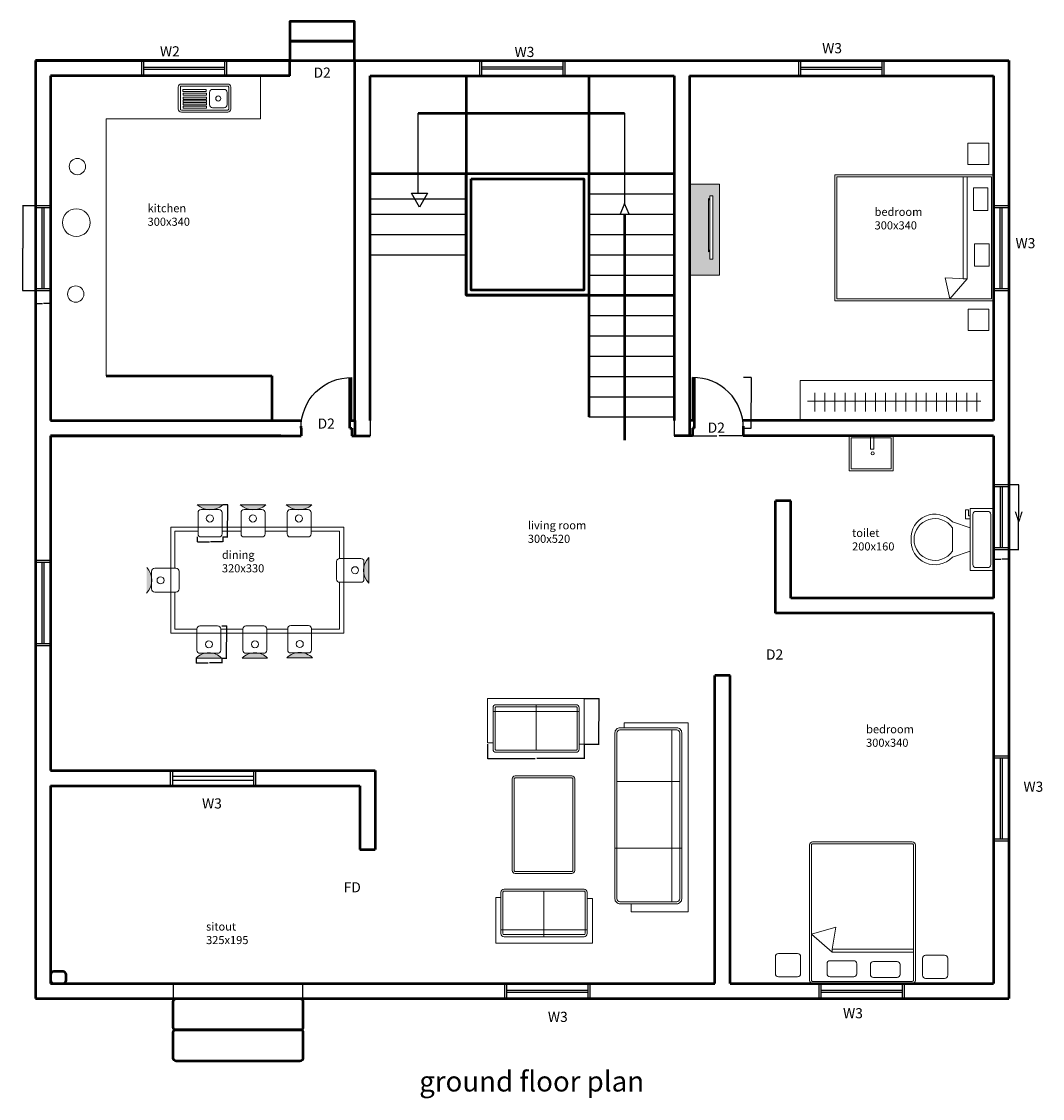
# Model space of a CAD drawing. Units: metres. Extents: x 10365 to 12529, y 3661 to 6248.
# Tile 1 of 9: x 10365 to 11372, y 3661 to 4723. Entities that reach past the tile are written whole.
import ezdxf

# ---------------------------------------------------------------- set-up
doc = ezdxf.new("R2010")
doc.units = ezdxf.units.M
doc.header["$MEASUREMENT"] = 0
for name, color, linetype, lineweight in [('A-ANNO-DIMS', 2, 'Continuous', 18), ('A-ANNO-TEXT', 7, 'Continuous', 18), ('A-AREA-IDEN', 7, 'Continuous', 18), ('A-DOOR', 4, 'Continuous', 25), ('A-ELEV-PATT', 8, 'Continuous', 13), ('A-FLOR-FIXT', 8, 'Continuous', 18), ('A-FLOR-STRS', 3, 'Continuous', 25), ('A-FURN', 30, 'Continuous', 18), ('A-GLAZ', 4, 'Continuous', 25), ('A-WALL', 7, 'Continuous', 50)]:
    doc.layers.add(name, color=color, linetype=linetype, lineweight=lineweight)
doc.styles.get("Standard").update_dxf_attribs({"font": 'arial.ttf'})
doc.dimstyles.get("Standard").update_dxf_attribs({"dimtxt": 0.18, "dimasz": 0.18, "dimexe": 0.18, "dimexo": 0.0625, "dimgap": 0.09, "dimtad": 0, "dimtih": 1, "dimtoh": 1, "dimdec": 0, "dimzin": 0, "dimdsep": 46, "dimtxsty": 'Standard', "dimcen": 0.09, "dimadec": 0, "dimazin": 0, "dimtfac": 1, "dimtdec": 0, "dimtofl": 0, "dimtmove": 0, "dimatfit": 3, "dimfxl": 1, "dimtolj": 1, "dimtzin": 0, "dimarcsym": 0})

# ---------------------------------------------------------------- blocks, each defined once
blk = doc.blocks.new('*U2')
for p, q in [((9.5, -6), (9.5, -2)), ((-10, -8.5), (-8, -8.5)), ((-10, -9.5), (-10, -8.5)), ((-7, -9.5), (-10, -9.5)), ((-8, -8.5), (-8, -8)), ((-7, -8), (-7, -9.5)), ((-4, -8), (-6, -14)), ((4, -8), (6, -14)), ((4, -14), (-4, -14))]:
    blk.add_line(p, q)
blk.add_lwpolyline([(10.5, -8), (10.5, 0), (-10.5, 0), (-10.5, -8)], close=True)
for points in [[(-9.5, -2), (-9.5, -6)], [(8.5, -1), (-8.5, -1)], [(-8.5, -7), (8.5, -7)]]:
    blk.add_lwpolyline(points)
for centre, radius, start, end in [((-8.625, -1.875), 0.8839, 81.8699, 188.1301), ((8.625, -1.875), 0.8839, 351.8699, 98.1301), ((-8.625, -6.125), 0.8839, 171.869898, 278.1301), ((8.625, -6.125), 0.8839, 261.8699, 8.1301), ((-0.4772, -19.9188), 8.0953, 133.01722, 273.38), ((0.0374, -19.8731), 7.127, 124.50543, 269.7), ((-0.0373, -19.8731), 7.127, 270.3, 55.4946), ((0.4773, -19.9188), 8.0953, 266.62, 46.9828)]:
    blk.add_arc(centre, radius, start, end)
blk = doc.blocks.new('CHAIR-A')
h = blk.add_hatch()
h.set_pattern_fill('ANSI38', color=256)
h.set_pattern_definition([(45, (-1779.3996, -783.2818), (-0.088388348, 0.088388348), []), (135, (-1779.3996, -783.2818), (-0.265165043, 0.088388348), [0.3125, -0.1875])])
h.paths.add_polyline_path([(25.2, 31.8), (19.1, 31.8), (0, 31.8, 0.145448), (8.9, 27), (16.3, 27, 0.145137)])
for p, q in [((0, 31.8), (25.2, 31.8)), ((25.2, 31.8), (19.1, 31.8)), ((19.1, 31.8), (25.2, 31.8))]:
    blk.add_line(p, q)
blk.add_lwpolyline([(0.9, 24, -0.414214), (3.9, 27), (21.5, 27, -0.414214), (24.5, 24), (24.5, 3, -0.414214), (21.5, 0), (3.9, 0, -0.414214), (0.9, 3)], format="xyb", close=True)
blk.add_circle((12.5, 18.2), 3.48)
blk.add_arc((12.6, 44.4), 17.8, 224.9651, 314.9651)
blk = doc.blocks.new('CHAIR-B')
h = blk.add_hatch()
h.set_pattern_fill('ANSI38', color=256, angle=180)
h.set_pattern_definition([(225, (1804.6167, 815.10581), (0.088388348, -0.088388348), []), (315, (1804.6167, 815.10581), (0.265165043, -0.088388348), [0.3125, -0.1875])])
h.paths.add_polyline_path([(8.9, 4.8, 0.145137), (0, 0), (6.1, 0), (25.2, 0, 0.145448), (16.3, 4.8)])
for p, q in [((0, 0), (6.1, 0)), ((6.1, 0), (0, 0)), ((25.2, 0), (0, 0))]:
    blk.add_line(p, q)
blk.add_lwpolyline([(24.3, 7.8, -0.414214), (21.3, 4.8), (3.8, 4.8, -0.414214), (0.8, 7.8), (0.8, 28.8, -0.414214), (3.8, 31.8), (21.3, 31.8, -0.414214), (24.3, 28.8)], format="xyb", close=True)
blk.add_circle((12.7, 13.6), 3.48)
blk.add_arc((12.6, -12.6), 17.8, 44.9651, 134.9651)
blk = doc.blocks.new('DOOR-D2')
blk.add_line((0, 7.5), (0, 50))
blk.add_arc((1, 1), 49, 358.8309, 91.1691)
blk = doc.blocks.new('SOFA-2SEAT')
for p, q in [((0, 1.2), (0, 45.1)), ((0, 45.1), (95.5, 45.1)), ((95.5, 45.1), (95.5, 0)), ((5.5, 1.2), (0, 1.2)), ((95.5, 0), (90.4, 0))]:
    blk.add_line(p, q)
blk = doc.blocks.new('WIN-800')
for p, q in [((0, 0), (0, 15)), ((2, 0), (2, 15)), ((82, 0), (82, 15)), ((84, 0), (84, 15)), ((2, 8.5), (82, 8.5)), ((2, 6.5), (82, 6.5))]:
    blk.add_line(p, q)
blk = doc.blocks.new('VENT-600')
for p, q in [((0, 64), (15, 64)), ((0, 62), (15, 62)), ((6.5, 62), (6.5, 2)), ((8.5, 62), (8.5, 2)), ((8.5, 62), (8.5, 2)), ((0, 2), (15, 2)), ((0, 0), (15, 0))]:
    blk.add_line(p, q)
blk = doc.blocks.new('WIN-800-B')
for p, q in [((0, 84), (15, 84)), ((0, 82), (15, 82)), ((6.5, 82), (6.5, 2)), ((8.5, 82), (8.5, 2)), ((8.5, 82), (8.5, 2)), ((0, 2), (15, 2)), ((0, 0), (15, 0))]:
    blk.add_line(p, q)
blk = doc.blocks.new('*D17')
at = {"layer": 'A-ANNO-DIMS', "color": 0, "lineweight": -2, "transparency": 16777216}
for p, q in [((10378.4, 4541.8), (10365.7, 4541.8)), ((10365.8, 4541.6), (10365.8, 4500)), ((10365.8, 4458), (10365.8, 4499.6)), ((10378.4, 4457.8), (10365.7, 4457.8))]:
    blk.add_line(p, q, dxfattribs=at)
at = {"layer": 'A-ANNO-DIMS', "color": 0, "transparency": 16777216}
for points in [[(10365.8, 4541.6), (10365.9, 4541.6), (10365.8, 4541.8)], [(10365.8, 4458), (10365.9, 4458), (10365.8, 4457.8)]]:
    blk.add_solid(points, dxfattribs=at)
at = {"layer": 'Defpoints', "color": 0, "transparency": 16777216}
for p in [(10365.8, 4541.8), (10378.4, 4541.8), (10378.4, 4457.8)]:
    blk.add_point(p, dxfattribs=at)
at = {"layer": 'A-ANNO-DIMS', "color": 0, "transparency": 16777216, "insert": (10365.8, 4499.8), "char_height": 0.18, "attachment_point": 5}
blk.add_mtext('\\A1;WINDOW W3 84 TYP.', dxfattribs=at)
blk = doc.blocks.new('*D18')
at = {"layer": 'A-ANNO-DIMS', "color": 0, "lineweight": -2, "transparency": 16777216}
for p, q in [((10378.4, 4457.8), (10378.4, 4445)), ((10393.4, 4457.8), (10393.4, 4445)), ((10378.6, 4445.2), (10385.4, 4445.2)), ((10393.3, 4445.2), (10386.5, 4445.2))]:
    blk.add_line(p, q, dxfattribs=at)
at = {"layer": 'A-ANNO-DIMS', "color": 0, "transparency": 16777216}
for points in [[(10378.6, 4445.2), (10378.6, 4445.2), (10378.4, 4445.2)], [(10393.3, 4445.2), (10393.3, 4445.2), (10393.4, 4445.2)]]:
    blk.add_solid(points, dxfattribs=at)
at = {"layer": 'Defpoints', "color": 0, "transparency": 16777216}
for p in [(10378.4, 4457.8), (10393.4, 4457.8), (10378.4, 4445.2)]:
    blk.add_point(p, dxfattribs=at)
at = {"layer": 'A-ANNO-DIMS', "color": 0, "transparency": 16777216, "insert": (10385.9, 4445.2), "char_height": 0.18, "attachment_point": 5}
blk.add_mtext('\\A1;15 TYP.', dxfattribs=at)
blk = doc.blocks.new('*D21')
at = {"layer": 'A-ANNO-DIMS', "color": 0, "lineweight": -2, "transparency": 16777216}
for p, q in [((11338.5, 4266.8), (11348.2, 4266.8)), ((11348, 4266.6), (11348, 4235)), ((11348, 4203), (11348, 4234.6)), ((11338.5, 4202.8), (11348.2, 4202.8))]:
    blk.add_line(p, q, dxfattribs=at)
at = {"layer": 'A-ANNO-DIMS', "color": 0, "transparency": 16777216}
for points in [[(11348, 4266.6), (11348.1, 4266.6), (11348, 4266.8)], [(11348, 4203), (11348.1, 4203), (11348, 4202.8)]]:
    blk.add_solid(points, dxfattribs=at)
at = {"layer": 'Defpoints', "color": 0, "transparency": 16777216}
for p in [(11338.4, 4266.8), (11348, 4266.8), (11338.4, 4202.8)]:
    blk.add_point(p, dxfattribs=at)
at = {"layer": 'A-ANNO-DIMS', "color": 0, "transparency": 16777216, "insert": (11348, 4234.8), "char_height": 0.18, "attachment_point": 5}
blk.add_mtext('\\A1;VENT V 64 TYP.', dxfattribs=at)
blk = doc.blocks.new('*D22')
at = {"layer": 'A-ANNO-DIMS', "color": 0, "lineweight": -2, "transparency": 16777216}
for p, q in [((11323.4, 4202.8), (11323.4, 4193)), ((11338.4, 4202.8), (11338.4, 4193)), ((11323.6, 4193.2), (11330.4, 4193.2)), ((11338.3, 4193.2), (11331.5, 4193.2))]:
    blk.add_line(p, q, dxfattribs=at)
at = {"layer": 'A-ANNO-DIMS', "color": 0, "transparency": 16777216}
for points in [[(11323.6, 4193.2), (11323.6, 4193.2), (11323.4, 4193.2)], [(11338.3, 4193.2), (11338.3, 4193.2), (11338.4, 4193.2)]]:
    blk.add_solid(points, dxfattribs=at)
at = {"layer": 'Defpoints', "color": 0, "transparency": 16777216}
for p in [(11323.4, 4202.8), (11338.4, 4202.8), (11338.4, 4193.2)]:
    blk.add_point(p, dxfattribs=at)
at = {"layer": 'A-ANNO-DIMS', "color": 0, "transparency": 16777216, "insert": (11330.9, 4193.2), "char_height": 0.18, "attachment_point": 5}
blk.add_mtext('\\A1;15 TYP.', dxfattribs=at)
blk = doc.blocks.new('*D23')
at = {"layer": 'A-ANNO-DIMS', "color": 0, "lineweight": -2, "transparency": 16777216}
for p, q in [((11026.4, 4322.3), (11026.4, 4314.6)), ((11026.6, 4314.8), (11050.4, 4314.8)), ((11076.5, 4314.8), (11052.7, 4314.8)), ((11076.7, 4322.3), (11076.7, 4314.6))]:
    blk.add_line(p, q, dxfattribs=at)
at = {"layer": 'A-ANNO-DIMS', "color": 0, "transparency": 16777216}
for points in [[(11026.6, 4314.8), (11026.6, 4314.7), (11026.4, 4314.8)], [(11076.5, 4314.8), (11076.5, 4314.7), (11076.7, 4314.8)]]:
    blk.add_solid(points, dxfattribs=at)
at = {"layer": 'Defpoints', "color": 0, "transparency": 16777216}
for p in [(11026.4, 4322.3), (11076.7, 4322.3), (11076.7, 4314.8)]:
    blk.add_point(p, dxfattribs=at)
at = {"layer": 'A-ANNO-DIMS', "color": 0, "transparency": 16777216, "insert": (11051.6, 4314.8), "char_height": 0.18, "attachment_point": 5}
blk.add_mtext('\\A1;DOOR D2 50 TYP.', dxfattribs=at)
blk = doc.blocks.new('*D24')
at = {"layer": 'A-ANNO-DIMS', "color": 0, "lineweight": -2, "transparency": 16777216}
for p, q in [((11076.8, 4372.6), (11084.4, 4372.6)), ((11084.2, 4372.4), (11084.2, 4347.6)), ((11084.2, 4322.5), (11084.2, 4347.3)), ((11076.8, 4322.3), (11084.4, 4322.3))]:
    blk.add_line(p, q, dxfattribs=at)
at = {"layer": 'A-ANNO-DIMS', "color": 0, "transparency": 16777216}
for points in [[(11084.2, 4372.4), (11084.3, 4372.4), (11084.2, 4372.6)], [(11084.2, 4322.5), (11084.3, 4322.5), (11084.2, 4322.3)]]:
    blk.add_solid(points, dxfattribs=at)
at = {"layer": 'Defpoints', "color": 0, "transparency": 16777216}
for p in [(11076.7, 4372.6), (11084.2, 4372.6), (11076.7, 4322.3)]:
    blk.add_point(p, dxfattribs=at)
at = {"layer": 'A-ANNO-DIMS', "color": 0, "transparency": 16777216, "insert": (11084.2, 4347.4), "char_height": 0.18, "attachment_point": 5}
blk.add_mtext('\\A1;50 TYP.', dxfattribs=at)
blk = doc.blocks.new('*D25')
at = {"layer": 'A-ANNO-DIMS', "color": 0, "lineweight": -2, "transparency": 16777216}
for p, q in [((10563.2, 4247), (10568, 4247)), ((10567.9, 4246.8), (10567.9, 4231.2)), ((10567.9, 4215.3), (10567.9, 4230.9)), ((10563.2, 4215.1), (10568, 4215.1))]:
    blk.add_line(p, q, dxfattribs=at)
at = {"layer": 'A-ANNO-DIMS', "color": 0, "transparency": 16777216}
for points in [[(10567.8, 4246.8), (10567.9, 4246.8), (10567.9, 4247)], [(10567.8, 4215.3), (10567.9, 4215.3), (10567.9, 4215.1)]]:
    blk.add_solid(points, dxfattribs=at)
at = {"layer": 'Defpoints', "color": 0, "transparency": 16777216}
for p in [(10563.1, 4247), (10567.9, 4247), (10563.1, 4215.1)]:
    blk.add_point(p, dxfattribs=at)
at = {"layer": 'A-ANNO-DIMS', "color": 0, "transparency": 16777216, "insert": (10567.9, 4231.1), "char_height": 0.18, "attachment_point": 5}
blk.add_mtext('\\A1;CHAIR A 32 TYP.', dxfattribs=at)
blk = doc.blocks.new('*D26')
at = {"layer": 'A-ANNO-DIMS', "color": 0, "lineweight": -2, "transparency": 16777216}
for p, q in [((10537.9, 4215.1), (10537.9, 4210.2)), ((10538.1, 4210.4), (10550, 4210.4)), ((10562.9, 4210.4), (10551, 4210.4)), ((10563.1, 4215.1), (10563.1, 4210.2))]:
    blk.add_line(p, q, dxfattribs=at)
at = {"layer": 'A-ANNO-DIMS', "color": 0, "transparency": 16777216}
for points in [[(10538.1, 4210.4), (10538.1, 4210.3), (10537.9, 4210.4)], [(10562.9, 4210.4), (10562.9, 4210.3), (10563.1, 4210.4)]]:
    blk.add_solid(points, dxfattribs=at)
at = {"layer": 'Defpoints', "color": 0, "transparency": 16777216}
for p in [(10537.9, 4215.1), (10563.1, 4215.1), (10563.1, 4210.4)]:
    blk.add_point(p, dxfattribs=at)
at = {"layer": 'A-ANNO-DIMS', "color": 0, "transparency": 16777216, "insert": (10550.5, 4210.4), "char_height": 0.18, "attachment_point": 5}
blk.add_mtext('\\A1;25 TYP.', dxfattribs=at)
blk = doc.blocks.new('*D27')
at = {"layer": 'A-ANNO-DIMS', "color": 0, "lineweight": -2, "transparency": 16777216}
for p, q in [((10562.1, 4127.4), (10567, 4127.4)), ((10566.8, 4127.3), (10566.8, 4111.7)), ((10566.8, 4095.8), (10566.8, 4111.3)), ((10562.1, 4095.6), (10567, 4095.6))]:
    blk.add_line(p, q, dxfattribs=at)
at = {"layer": 'A-ANNO-DIMS', "color": 0, "transparency": 16777216}
for points in [[(10566.8, 4127.3), (10566.9, 4127.3), (10566.8, 4127.4)], [(10566.8, 4095.8), (10566.9, 4095.8), (10566.8, 4095.6)]]:
    blk.add_solid(points, dxfattribs=at)
at = {"layer": 'Defpoints', "color": 0, "transparency": 16777216}
for p in [(10562.1, 4127.4), (10566.8, 4127.4), (10562.1, 4095.6)]:
    blk.add_point(p, dxfattribs=at)
at = {"layer": 'A-ANNO-DIMS', "color": 0, "transparency": 16777216, "insert": (10566.8, 4111.5), "char_height": 0.18, "attachment_point": 5}
blk.add_mtext('\\A1;CHAIR B 32 TYP.', dxfattribs=at)
blk = doc.blocks.new('*D28')
at = {"layer": 'A-ANNO-DIMS', "color": 0, "lineweight": -2, "transparency": 16777216}
for p, q in [((10536.8, 4095.6), (10536.8, 4090.7)), ((10537, 4090.8), (10548.9, 4090.8)), ((10561.9, 4090.8), (10550, 4090.8)), ((10562.1, 4095.6), (10562.1, 4090.7))]:
    blk.add_line(p, q, dxfattribs=at)
at = {"layer": 'A-ANNO-DIMS', "color": 0, "transparency": 16777216}
for points in [[(10537, 4090.9), (10537, 4090.8), (10536.8, 4090.8)], [(10561.9, 4090.9), (10561.9, 4090.8), (10562.1, 4090.8)]]:
    blk.add_solid(points, dxfattribs=at)
at = {"layer": 'Defpoints', "color": 0, "transparency": 16777216}
for p in [(10536.8, 4095.6), (10562.1, 4095.6), (10562.1, 4090.8)]:
    blk.add_point(p, dxfattribs=at)
at = {"layer": 'A-ANNO-DIMS', "color": 0, "transparency": 16777216, "insert": (10549.5, 4090.8), "char_height": 0.18, "attachment_point": 5}
blk.add_mtext('\\A1;25 TYP.', dxfattribs=at)
blk = doc.blocks.new('*D29')
at = {"layer": 'A-ANNO-DIMS', "color": 0, "lineweight": -2, "transparency": 16777216}
for p, q in [((10824.2, 4010.7), (10824.2, 3996.3)), ((10919.7, 4010.7), (10919.7, 3996.3)), ((10824.4, 3996.5), (10871.1, 3996.5)), ((10919.5, 3996.5), (10872.9, 3996.5))]:
    blk.add_line(p, q, dxfattribs=at)
at = {"layer": 'A-ANNO-DIMS', "color": 0, "transparency": 16777216}
for points in [[(10824.4, 3996.5), (10824.4, 3996.5), (10824.2, 3996.5)], [(10919.5, 3996.5), (10919.5, 3996.5), (10919.7, 3996.5)]]:
    blk.add_solid(points, dxfattribs=at)
at = {"layer": 'Defpoints', "color": 0, "transparency": 16777216}
for p in [(10824.2, 4010.8), (10919.7, 4010.8), (10919.7, 3996.5)]:
    blk.add_point(p, dxfattribs=at)
at = {"layer": 'A-ANNO-DIMS', "color": 0, "transparency": 16777216, "insert": (10872, 3996.5), "char_height": 0.18, "attachment_point": 5}
blk.add_mtext('\\A1;SOFA 96 TYP.', dxfattribs=at)
blk = doc.blocks.new('*D30')
at = {"layer": 'A-ANNO-DIMS', "color": 0, "lineweight": -2, "transparency": 16777216}
for p, q in [((10919.8, 4055.9), (10934.2, 4055.9)), ((10934, 4055.7), (10934, 4033.5)), ((10934, 4011), (10934, 4033.2)), ((10919.8, 4010.8), (10934.2, 4010.8))]:
    blk.add_line(p, q, dxfattribs=at)
at = {"layer": 'A-ANNO-DIMS', "color": 0, "transparency": 16777216}
for points in [[(10934, 4055.7), (10934.1, 4055.7), (10934, 4055.9)], [(10934, 4011), (10934.1, 4011), (10934, 4010.8)]]:
    blk.add_solid(points, dxfattribs=at)
at = {"layer": 'Defpoints', "color": 0, "transparency": 16777216}
for p in [(10919.7, 4055.9), (10934, 4055.9), (10919.7, 4010.8)]:
    blk.add_point(p, dxfattribs=at)
at = {"layer": 'A-ANNO-DIMS', "color": 0, "transparency": 16777216, "insert": (10934, 4033.4), "char_height": 0.18, "attachment_point": 5}
blk.add_mtext('\\A1;45 TYP.', dxfattribs=at)

msp = doc.modelspace()

# ---------------------------------------------------------------- hatches: boundary and pattern name
at = {"layer": 'A-ELEV-PATT'}
h = msp.add_hatch(dxfattribs=at)
h.set_pattern_fill('ANSI38', color=256, angle=450)
h.set_pattern_definition([(135, (11303.24476, 2380.41181), (-0.088388348, -0.088388348), []), (225, (11303.24476, 2380.41181), (-0.088388348, -0.265165043), [0.3125, -0.1875])])
h.paths.add_polyline_path([(10493, 4176.1, 0.145137), (10488.2, 4185), (10488.2, 4178.9), (10488.1, 4159.8, 0.145448), (10493, 4168.7)])
at = {"layer": 'A-FURN'}
h = msp.add_hatch(color=256, dxfattribs=at)
h.dxf.hatch_style = 1
h.paths.add_polyline_path([(11052.9, 4563.1), (11023.4, 4563.1), (11023.4, 4473.3), (11052.9, 4473.3)])
h.paths.add_polyline_path([(11043.5, 4547.2), (11042.1, 4548.9), (11042.1, 4496.2), (11043.5, 4498.3)], flags=16)
h.paths.add_polyline_path([(11046.3, 4551.4), (11043.5, 4551.4), (11043.5, 4489.2), (11046.3, 4489.2)], flags=16)

# ---------------------------------------------------------------- linework, layer by layer
at = {"layer": 'A-FLOR-FIXT'}
for p, q in [((10600.2, 4669.8), (10600.2, 4627.3)), ((10600.2, 4627.3), (10448.1, 4627.3)), ((10448.1, 4627.3), (10448.1, 4374))]:
    msp.add_line(p, q, dxfattribs=at)
for points in [[(10521.3, 4658.7, -0.414214), (10522.3, 4659.7), (10568, 4659.7, -0.414214), (10569, 4658.7), (10569, 4637.1, -0.414214), (10568, 4636.1), (10522.3, 4636.1, -0.414214), (10521.3, 4637.1)], [(10550.1, 4653.5, -0.414214), (10553.1, 4656.5), (10564.4, 4656.5, -0.414214), (10567.4, 4653.5), (10567.4, 4641.4, -0.414214), (10564.4, 4638.4), (10553.1, 4638.4, -0.414214), (10550.1, 4641.4)]]:
    msp.add_lwpolyline(points, format="xyb", close=True, dxfattribs=at)
for points in [[(10523.6, 4656.5), (10523.6, 4656.5), (10546.7, 4656.5), (10546.7, 4656.5), (10546.7, 4654.4), (10546.7, 4654.4), (10523.6, 4654.4), (10523.6, 4654.4)], [(10524.2, 4652.7), (10524.2, 4652.7), (10547.2, 4652.7), (10547.2, 4652.7), (10547.2, 4650.7), (10547.2, 4650.7), (10524.2, 4650.7), (10524.2, 4650.7)], [(10524.2, 4648.9), (10524.2, 4648.9), (10547.2, 4648.9), (10547.2, 4648.9), (10547.2, 4646.8), (10547.2, 4646.8), (10524.2, 4646.8), (10524.2, 4646.8)], [(10524.2, 4645.9), (10524.2, 4645.9), (10547.2, 4645.9), (10547.2, 4645.9), (10547.2, 4643.9), (10547.2, 4643.9), (10524.2, 4643.9), (10524.2, 4643.9)], [(10524.2, 4643.2), (10524.2, 4643.2), (10547.2, 4643.2), (10547.2, 4643.2), (10547.2, 4641.2), (10547.2, 4641.2), (10524.2, 4641.2), (10524.2, 4641.2)], [(10524.2, 4639.8), (10524.2, 4639.8), (10547.2, 4639.8), (10547.2, 4639.8), (10547.2, 4637.8), (10547.2, 4637.8), (10524.2, 4637.8), (10524.2, 4637.8)], [(11181, 4314.8), (11224.3, 4314.8), (11224.3, 4280.3), (11181, 4280.3)], [(11183, 4312.8), (11222.3, 4312.8), (11222.3, 4282.3), (11183, 4282.3)], [(11205.4, 4314.8), (11202, 4314.8), (11202, 4301.7), (11205.4, 4301.7)]]:
    msp.add_lwpolyline(points, close=True, dxfattribs=at)
for centre, radius in [((10558.7, 4647.5), 2.48), ((10419.8, 4580.4), 8.05), ((10418.7, 4525.1), 13.6), ((10418.1, 4454.6), 8.05), ((11204.1, 4297.5), 1.49)]:
    msp.add_circle(centre, radius, dxfattribs=at)
at = {"layer": 'A-FLOR-STRS'}
for p, q in [((10755.8, 4554), (10755.8, 4633)), ((10959.2, 4633), (10959.2, 4543.9)), ((10708.4, 4548.4), (10803.2, 4548.4)), ((10749.4, 4554), (10765.2, 4554)), ((10757.3, 4540.3), (10749.4, 4554)), ((10765.2, 4554), (10757.3, 4540.3)), ((10924.3, 4553.4), (11008.4, 4553.4)), ((10959.2, 4543.9), (10955, 4533.4)), ((10963.8, 4533.4), (10959.2, 4543.9)), ((10708.4, 4533.4), (10803.2, 4533.4)), ((10924.3, 4533.4), (11008.4, 4533.4)), ((10959.2, 4533.4), (10963.8, 4533.4)), ((10708.4, 4513.4), (10803.2, 4513.4)), ((10924.3, 4513.4), (11008.4, 4513.4)), ((10708.4, 4493.4), (10803.2, 4493.4)), ((10924.3, 4493.4), (11008.4, 4493.4)), ((10924.3, 4473.4), (11008.4, 4473.4)), ((10924.3, 4433.4), (11008.4, 4433.4)), ((10924.3, 4413.4), (11008.4, 4413.4)), ((10924.3, 4393.4), (11008.4, 4393.4)), ((10924.3, 4373.4), (11008.4, 4373.4)), ((10924.3, 4353.4), (11008.4, 4353.4)), ((10924.3, 4333.4), (11008.4, 4333.4)), ((10708.4, 4329.8), (10708.4, 4314.8)), ((11008.4, 4329.8), (11008.4, 4314.8)), ((10514.2, 3774.8), (10514.2, 3759.8)), ((10641.8, 3774.8), (10641.8, 3759.8))]:
    msp.add_line(p, q, dxfattribs=at)
at = {"layer": 'A-FURN'}
for p, q in [((11043.5, 4547.2), (11042.1, 4548.9)), ((11042.1, 4548.9), (11042.1, 4496.2)), ((11042.1, 4496.2), (11043.5, 4498.3)), ((11280.3, 4449.8), (11275.6, 4470.7)), ((11275.6, 4470.7), (11297.3, 4469.7)), ((11297.3, 4469.7), (11280.3, 4449.8)), ((11132.6, 4329.8), (11132.6, 4369.4)), ((11132.6, 4369.4), (11323.4, 4369.4)), ((11146.9, 4357.2), (11146.9, 4338.8)), ((11156.9, 4357.2), (11156.9, 4338.8)), ((11166.9, 4357.2), (11166.9, 4338.8)), ((11176.9, 4357.2), (11176.9, 4338.8)), ((11186.9, 4357.2), (11186.9, 4338.8)), ((11196.9, 4357.2), (11196.9, 4338.8)), ((11206.9, 4357.2), (11206.9, 4338.8)), ((11216.9, 4357.2), (11216.9, 4338.8)), ((11226.9, 4357.2), (11226.9, 4338.8)), ((11236.9, 4357.2), (11236.9, 4338.8)), ((11246.9, 4357.2), (11246.9, 4338.8)), ((11256.9, 4357.2), (11256.9, 4338.8)), ((11266.9, 4357.2), (11266.9, 4338.8)), ((11276.9, 4357.2), (11276.9, 4338.8)), ((11286.9, 4357.2), (11286.9, 4338.8)), ((11296.9, 4357.2), (11296.9, 4338.8)), ((11306.9, 4357.2), (11306.9, 4338.8)), ((11139.9, 4349), (11310.8, 4349)), ((10872.1, 4049.6), (10872.1, 4004.7)), ((10829.7, 4042.8), (10914.6, 4042.8)), ((10959.1, 4026.9), (10959.1, 4031.8)), ((10959.1, 4031.8), (11022, 4031.8)), ((11022, 4031.8), (11022, 3845.3)), ((11006.1, 4024.9), (11006.1, 3855.3)), ((10951.9, 3973.9), (11013.8, 3973.9)), ((10949.9, 3908.1), (11015.8, 3908.1)), ((10879.9, 3820.9), (10879.9, 3865.7)), ((10966, 3845.3), (10966, 3853.3)), ((11022, 3845.3), (10966, 3845.3)), ((10922.4, 3827.6), (10837.5, 3827.6)), ((11143.8, 3823.3), (11167.8, 3830.4)), ((11167.8, 3830.4), (11164.2, 3808.7)), ((11164.2, 3805.6), (11143.8, 3823.3))]:
    msp.add_line(p, q, dxfattribs=at)
for points in [[(10519.3, 4658.7, -0.414214), (10522.3, 4661.7), (10568, 4661.7, -0.414214), (10571, 4658.7), (10571, 4637.1, -0.414214), (10568, 4634.1), (10522.3, 4634.1, -0.414214), (10519.3, 4637.1)], [(10496, 4160.8, -0.414214), (10493, 4163.8), (10493, 4181.3, -0.414214), (10496, 4184.3), (10517, 4184.3, -0.414214), (10520, 4181.3), (10520, 4163.8, -0.414214), (10517, 4160.8)], [(10829.7, 4046.6, -0.414214), (10832.7, 4049.6), (10911.6, 4049.6, -0.414214), (10914.6, 4046.6), (10914.6, 4005.7, -0.414214), (10911.6, 4002.7), (10832.7, 4002.7, -0.414214), (10829.7, 4005.7)], [(10831.7, 4046.6, -0.414214), (10832.7, 4047.6), (10911.6, 4047.6, -0.414214), (10912.6, 4046.6), (10912.6, 4005.7, -0.414214), (10911.6, 4004.7), (10832.7, 4004.7, -0.414214), (10831.7, 4005.7)], [(11015.8, 4021.9, 0.414214), (11010.8, 4026.9), (10954.9, 4026.9, 0.414214), (10949.9, 4021.9), (10949.9, 3858.3, 0.414214), (10954.9, 3853.3), (11010.8, 3853.3, 0.414214), (11015.8, 3858.3)], [(11013.8, 4021.9, 0.414214), (11010.8, 4024.9), (10954.9, 4024.9, 0.414214), (10951.9, 4021.9), (10951.9, 3858.3, 0.414214), (10954.9, 3855.3), (11010.8, 3855.3, 0.414214), (11013.8, 3858.3)], [(10848.5, 3976.4, -0.414214), (10851.5, 3979.4), (10907.4, 3979.4, -0.414214), (10910.4, 3976.4), (10910.4, 3886.2, -0.414214), (10907.4, 3883.2), (10851.5, 3883.2, -0.414214), (10848.5, 3886.2)], [(10850.5, 3976.4, -0.414214), (10851.5, 3977.4), (10907.4, 3977.4, -0.414214), (10908.4, 3976.4), (10908.4, 3886.2, -0.414214), (10907.4, 3885.2), (10851.5, 3885.2, -0.414214), (10850.5, 3886.2)], [(11246.2, 3777.8, -0.414214), (11243.2, 3774.8), (11144.8, 3774.8, -0.414214), (11141.8, 3777.8), (11141.8, 3911.4, -0.414214), (11144.8, 3914.4), (11243.2, 3914.4, -0.414214), (11246.2, 3911.4)], [(11244.2, 3777.8, -0.414214), (11243.2, 3776.8), (11144.8, 3776.8, -0.414214), (11143.8, 3777.8), (11143.8, 3911.4, -0.414214), (11144.8, 3912.4), (11243.2, 3912.4, -0.414214), (11244.2, 3911.4)], [(10922.4, 3823.9, -0.414214), (10919.4, 3820.9), (10840.5, 3820.9, -0.414214), (10837.5, 3823.9), (10837.5, 3864.7, -0.414214), (10840.5, 3867.7), (10919.4, 3867.7, -0.414214), (10922.4, 3864.7)], [(10920.4, 3823.9, -0.414214), (10919.4, 3822.9), (10840.5, 3822.9, -0.414214), (10839.5, 3823.9), (10839.5, 3864.7, -0.414214), (10840.5, 3865.7), (10919.4, 3865.7, -0.414214), (10920.4, 3864.7)], [(11108.1, 3801.3, -0.414214), (11111.1, 3804.3), (11130, 3804.3, -0.414214), (11133, 3801.3), (11133, 3784.4, -0.414214), (11130, 3781.4), (11111.1, 3781.4, -0.414214), (11108.1, 3784.4)], [(11253.2, 3799.7, -0.414214), (11256.2, 3802.7), (11275.1, 3802.7, -0.414214), (11278.1, 3799.7), (11278.1, 3782.8, -0.414214), (11275.1, 3779.8), (11256.2, 3779.8, -0.414214), (11253.2, 3782.8)], [(11159.1, 3794.2, -0.414214), (11162.1, 3797.2), (11185.4, 3797.2, -0.414214), (11188.4, 3794.2), (11188.4, 3784.4, -0.414214), (11185.4, 3781.4), (11162.1, 3781.4, -0.414214), (11159.1, 3784.4)], [(11201.8, 3793.4, -0.414214), (11204.8, 3796.4), (11228.1, 3796.4, -0.414214), (11231.1, 3793.4), (11231.1, 3783.6, -0.414214), (11228.1, 3780.6), (11204.8, 3780.6, -0.414214), (11201.8, 3783.6)]]:
    msp.add_lwpolyline(points, format="xyb", close=True, dxfattribs=at)
for points in [[(11298.1, 4603.3), (11318.7, 4603.3), (11318.7, 4582.4), (11298.1, 4582.4)], [(11323.4, 4572.3), (11166.7, 4572.3), (11166.7, 4447.8), (11323.4, 4447.8)], [(11321.4, 4570.3), (11168.7, 4570.3), (11168.7, 4449.8), (11321.4, 4449.8)], [(11293.4, 4570.3), (11297.3, 4570.3), (11297.3, 4469.7), (11293.4, 4469.7)], [(11023.4, 4563.1), (11052.9, 4563.1), (11052.9, 4473.3), (11023.4, 4473.3)], [(11303.4, 4559.3), (11317.8, 4559.3), (11317.8, 4537.1), (11303.4, 4537.1)], [(11043.5, 4551.4), (11046.3, 4551.4), (11046.3, 4489.2), (11043.5, 4489.2)], [(11304.5, 4504.3), (11318.9, 4504.3), (11318.9, 4482.1), (11304.5, 4482.1)], [(11298.3, 4439.7), (11318.8, 4439.7), (11318.8, 4418.8), (11298.3, 4418.8)], [(10511.9, 4224.8), (10682.4, 4224.8), (10682.4, 4120.2), (10511.9, 4120.2)], [(11244.2, 3805.6), (11244.2, 3805.6), (11164.2, 3805.6), (11164.2, 3805.6), (11164.2, 3808.7), (11164.2, 3808.7), (11244.2, 3808.7), (11244.2, 3808.7)]]:
    msp.add_lwpolyline(points, close=True, dxfattribs=at)
for points in [[(10515.9, 4184.3), (10515.9, 4220.8), (10538.8, 4220.8)], [(10562.3, 4220.8), (10581.3, 4220.8)], [(10604.8, 4220.8), (10626.7, 4220.8)], [(10650.2, 4220.8), (10678.4, 4220.8), (10678.4, 4193.8)], [(10678.4, 4170.3), (10678.4, 4124.2), (10650.7, 4124.2)], [(10537.6, 4124.2), (10515.9, 4124.2), (10515.9, 4160.8)], [(10583, 4124.2), (10561.1, 4124.2)], [(10627.2, 4124.2), (10606.5, 4124.2)]]:
    msp.add_lwpolyline(points, dxfattribs=at)
msp.add_circle((10501.8, 4172.3), 3.48, dxfattribs=at)
msp.add_arc((10475.5, 4172.4), 17.8, 314.9651, 44.9651, dxfattribs=at)
at = {"layer": 'A-GLAZ'}
for p, q in [((10511.4, 3984.8), (10511.4, 3969.8)), ((10513.4, 3984.8), (10513.4, 3969.8)), ((10593.4, 3984.8), (10593.4, 3969.8)), ((10595.4, 3984.8), (10595.4, 3969.8)), ((10513.4, 3979.3), (10593.4, 3979.3)), ((10513.4, 3975.3), (10593.4, 3975.3))]:
    msp.add_line(p, q, dxfattribs=at)
at = {"layer": 'A-WALL'}
for p, q in [((10629.2, 4684.8), (10378.4, 4684.8)), ((10378.4, 4684.8), (10378.4, 4329.8)), ((10378.4, 4684.8), (10629.2, 4684.8)), ((10629.2, 4669.8), (10629.2, 4684.8)), ((10693.4, 4669.8), (10693.4, 4684.8)), ((10693.4, 4684.8), (11338.4, 4684.8)), ((10708.4, 4684.8), (11008.4, 4684.8)), ((11338.4, 4684.8), (11338.4, 3759.8)), ((10629.2, 4669.8), (10393.4, 4669.8)), ((10393.4, 4669.8), (10393.4, 4329.8)), ((10693.4, 4329.8), (10693.4, 4669.8)), ((10708.4, 4329.8), (10708.4, 4669.8)), ((10708.4, 4669.8), (11008.4, 4669.8)), ((10803.2, 4669.8), (10803.2, 4453.4)), ((10924.3, 4669.8), (10924.3, 4333.4)), ((11008.4, 4669.8), (11008.4, 4329.8)), ((11023.4, 4669.8), (11023.4, 4329.8)), ((11023.4, 4669.8), (11323.4, 4669.8)), ((11323.4, 4669.8), (11323.4, 4329.8)), ((10755.8, 4633), (10959.2, 4633)), ((10708.4, 4573.4), (11008.4, 4573.4)), ((10959.2, 4533.4), (10959.2, 4310.4)), ((10803.2, 4453.4), (11008.4, 4453.4)), ((10448.1, 4374), (10611.6, 4374)), ((10611.6, 4374), (10611.6, 4329.8)), ((10688.4, 4322.3), (10688.4, 4372.3)), ((11028.4, 4322.3), (11028.4, 4372.3)), ((10378.4, 4329.8), (10378.4, 4314.8)), ((10393.4, 4329.8), (10620.5, 4329.8)), ((10620.5, 4329.8), (10640.9, 4329.8)), ((10640.4, 4322.3), (10640.4, 4324.3)), ((10688.4, 4329.8), (10693.4, 4329.8)), ((10693.4, 4329.8), (10693.4, 4314.8)), ((11023.4, 4329.8), (11023.4, 4314.8)), ((11028.4, 4329.8), (11023.4, 4329.8)), ((11323.4, 4329.8), (11076, 4329.8)), ((11076.4, 4324.3), (11076.4, 4314.8)), ((10378.4, 4314.8), (10378.4, 3984.8)), ((10393.4, 4314.8), (10620.5, 4314.8)), ((10393.4, 4314.8), (10393.4, 3984.8)), ((10620.5, 4314.8), (10393.4, 4314.8)), ((10620.5, 4314.8), (10640.4, 4314.8)), ((10640.4, 4322.3), (10640.4, 4314.8)), ((10688.4, 4322.3), (10690.4, 4322.3)), ((10690.4, 4322.3), (10690.4, 4314.8)), ((10690.4, 4314.8), (10693.4, 4314.8)), ((10693.4, 4314.8), (10708.4, 4314.8)), ((11026.4, 4314.8), (11008.4, 4314.8)), ((11026.4, 4322.3), (11026.4, 4314.8)), ((11028.4, 4322.3), (11026.4, 4322.3)), ((11323.4, 4314.8), (11076.4, 4314.8)), ((11323.4, 4314.8), (11323.4, 4154.8)), ((11338.4, 4314.8), (11338.4, 3759.8)), ((11108.4, 4139.8), (11108.4, 4250.7)), ((11123.4, 4250.7), (11108.4, 4250.7)), ((11123.4, 4154.8), (11123.4, 4250.7)), ((11323.4, 4154.8), (11123.4, 4154.8)), ((11323.4, 4139.8), (11108.4, 4139.8)), ((11323.4, 4139.8), (11323.4, 3774.8)), ((11338.4, 4139.8), (11338.4, 3759.8)), ((11048.4, 3774.8), (11048.4, 4078.4)), ((11063.4, 4078.4), (11048.4, 4078.4)), ((11063.4, 3774.8), (11063.4, 4078.4)), ((10378.4, 3984.8), (10378.4, 3969.8)), ((10393.4, 3984.8), (10713.4, 3984.8)), ((10713.4, 3984.8), (10713.4, 3906.8)), ((10378.4, 3969.8), (10378.4, 3759.8)), ((10393.4, 3969.8), (10698.4, 3969.8)), ((10393.4, 3969.8), (10393.4, 3774.8)), ((10698.4, 3969.8), (10698.4, 3906.8)), ((10698.4, 3906.8), (10713.4, 3906.8)), ((10393.4, 3774.8), (10718.4, 3774.8)), ((10718.4, 3774.8), (11048.4, 3774.8)), ((11063.4, 3774.8), (11323.4, 3774.8)), ((10378.4, 3759.8), (10718.4, 3759.8)), ((10378.4, 3759.8), (11338.4, 3759.8)), ((10718.4, 3759.8), (11048.4, 3759.8))]:
    msp.add_line(p, q, dxfattribs=at)
for points in [[(10629.2, 4704.1), (10692.9, 4704.1), (10692.9, 4723.4), (10629.2, 4723.4)], [(10629.2, 4684.8), (10692.9, 4684.8), (10692.9, 4704.1), (10629.2, 4704.1)], [(10803.2, 4573.4), (10924.3, 4573.4), (10924.3, 4453.4), (10803.2, 4453.4)], [(10808.2, 4568.4), (10919.3, 4568.4), (10919.3, 4458.4), (10808.2, 4458.4)]]:
    msp.add_lwpolyline(points, close=True, dxfattribs=at)
msp.add_lwpolyline([(10803.2, 4453.4), (10803.2, 4573.4), (10924.3, 4573.4), (10924.3, 4413.4)], dxfattribs=at)
for points in [[(10393.4, 3777.8, 0.414214), (10396.4, 3774.8), (10405.7, 3774.8, 0.414214), (10408.7, 3777.8), (10408.7, 3783.5, 0.414214), (10405.7, 3786.5), (10396.4, 3786.5, 0.414214), (10393.4, 3783.5)], [(10514.2, 3756.8, -0.414214), (10517.2, 3759.8), (10639.2, 3759.8, -0.414214), (10642.2, 3756.8), (10642.2, 3731.6, -0.414214), (10639.2, 3728.6), (10517.2, 3728.6, -0.414214), (10514.2, 3731.6)], [(10514.2, 3726.5, -0.414214), (10517.2, 3729.5), (10639.2, 3729.5, -0.414214), (10642.2, 3726.5), (10642.2, 3701.2, -0.414214), (10639.2, 3698.2), (10517.2, 3698.2, -0.414214), (10514.2, 3701.2)]]:
    msp.add_lwpolyline(points, format="xyb", close=True, dxfattribs=at)

# ---------------------------------------------------------------- block references
at = {"layer": 'A-DOOR', "extrusion": (0, 0, -1), "zscale": -1}
msp.add_blockref('DOOR-D2', (-10690.4, 4322.3), dxfattribs=at)
at = {"layer": 'A-DOOR'}
msp.add_blockref('DOOR-D2', (11026.4, 4322.3), dxfattribs=at)
at = {"layer": 'A-FLOR-FIXT', "xscale": 2.907913259437767, "yscale": 2.907913259437767, "zscale": 2.907913259437767, "rotation": 270}
msp.add_blockref('*U2', (11323.4, 4212.6), dxfattribs=at)
at = {"layer": 'A-FURN'}
for name, p in [('CHAIR-A', (10537.9, 4215.1)), ('CHAIR-A', (10580.3, 4215.1)), ('CHAIR-A', (10625.7, 4215.1)), ('CHAIR-B', (10536.8, 4095.6)), ('CHAIR-B', (10582.2, 4095.6)), ('CHAIR-B', (10626.4, 4095.9)), ('SOFA-2SEAT', (10824.2, 4010.8))]:
    msp.add_blockref(name, p, dxfattribs=at)
for name, p, rotation in [('CHAIR-B', (10707.2, 4169.6), 89.99999999999093), ('SOFA-2SEAT', (10927.9, 3859.6), 180)]:
    msp.add_blockref(name, p, dxfattribs=dict(at, rotation=rotation))
at = {"layer": 'A-GLAZ'}
for name, p in [('WIN-800', (10483.3, 4669.8)), ('WIN-800', (11131.4, 4669.8)), ('VENT-600', (11323.4, 4202.8)), ('WIN-800-B', (11323.4, 3915.3)), ('WIN-800', (10841.4, 3759.8)), ('WIN-800', (11151.4, 3759.8))]:
    msp.add_blockref(name, p, dxfattribs=at)
for p, rotation in [((10900.4, 4684.8), 180), ((10393.4, 4457.8), 89.99999999999653), ((11338.4, 4457.8), 89.99999999999412), ((10393.4, 4107.8), 89.99999999999653)]:
    msp.add_blockref('WIN-800', p, dxfattribs=dict(at, rotation=rotation))

# ---------------------------------------------------------------- texts
at = {"layer": 'A-ANNO-TEXT', "attachment_point": 1}
for s, width, insert, char_height in [('W2', 63.407, (10501.2, 4699), 10), ('W3', 63.407, (10850.9, 4698.4), 10), ('W3', 63.407, (11154.3, 4702.1), 10), ('D2', 63.407, (10652.7, 4678), 10), ('W3', 63.407, (11345, 4509.8), 10), ('D2', 63.407, (10656.7, 4331.9), 10), ('D2', 63.407, (11041.4, 4327.9), 10), ('V', 63.407, (11344.2, 4240.1), 10), ('D2', 63.407, (11098.9, 4104.2), 10), ('W3', 63.407, (11352.8, 3973.8), 10), ('W3', 63.407, (10542.7, 3957.3), 10), ('FD', 63.407, (10682.4, 3874.6), 10), ('W3', 63.407, (11174.9, 3750.4), 10), ('W3', 63.407, (10883.8, 3746.8), 10), ('ground floor plan', 412.275, (10756.9, 3688.2), 20)]:
    msp.add_mtext_dynamic_manual_height_columns(s, width=width, gutter_width=1, heights=[0], dxfattribs=dict(at, insert=insert, char_height=char_height))
at = {"layer": 'A-AREA-IDEN', "char_height": 8, "attachment_point": 1}
for s, insert in [('kitchen\\P300x340', (10489, 4543.3)), ('bedroom\\P300x340', (11206, 4539.7)), ('living room\\P300x520', (10864, 4230.6)), ('toilet\\P200x160', (11183.8, 4223.1)), ('dining\\P320x330', (10562.3, 4201.5)), ('bedroom\\P300x340', (11197.6, 4029.5)), ('sitout\\P325x195', (10546.7, 3834.9))]:
    msp.add_mtext_dynamic_manual_height_columns(s, width=106.401, gutter_width=1, heights=[0], dxfattribs=dict(at, insert=insert))

# ---------------------------------------------------------------- dimensions: what is measured, and where the dimension line sits
at = {"layer": 'A-ANNO-DIMS'}
for base, p1, p2, angle, text, picture, middle in [((10365.8, 4541.8), (10378.4, 4457.8), (10378.4, 4541.8), 90, 'WINDOW W3 <> TYP.', '*D17', (10365.8, 4499.8)), ((10378.4, 4445.2), (10393.4, 4457.8), (10378.4, 4457.8), 180, '<> TYP.', '*D18', (10385.9, 4445.2)), ((11084.2, 4372.6), (11076.7, 4322.3), (11076.7, 4372.6), 90, '<> TYP.', '*D24', (11084.2, 4347.4)), ((11348, 4266.8), (11338.4, 4202.8), (11338.4, 4266.8), 90, 'VENT V <> TYP.', '*D21', (11348, 4234.8)), ((10567.9, 4247), (10563.1, 4215.1), (10563.1, 4247), 90, 'CHAIR A <> TYP.', '*D25', (10567.9, 4231.1)), ((10566.8, 4127.4), (10562.1, 4095.6), (10562.1, 4127.4), 90, 'CHAIR B <> TYP.', '*D27', (10566.8, 4111.5)), ((10934, 4055.9), (10919.7, 4010.8), (10919.7, 4055.9), 90, '<> TYP.', '*D30', (10934, 4033.4))]:
    dim = msp.add_linear_dim(base=base, p1=p1, p2=p2, angle=angle, text=text, dimstyle='Standard', override={"dimdec": 0, "dimrnd": 0, "dimzin": 0, "dimlunit": 2}, dxfattribs=at)
    dim.commit()
    dim.dimension.update_dxf_attribs({"geometry": picture, "text_midpoint": middle})
for base, p1, p2, text, picture, middle in [((11076.7, 4314.8), (11026.4, 4322.3), (11076.7, 4322.3), 'DOOR D2 <> TYP.', '*D23', (11051.6, 4314.8)), ((10563.1, 4210.4), (10537.9, 4215.1), (10563.1, 4215.1), '<> TYP.', '*D26', (10550.5, 4210.4)), ((11338.4, 4193.2), (11323.4, 4202.8), (11338.4, 4202.8), '<> TYP.', '*D22', (11330.9, 4193.2)), ((10562.1, 4090.8), (10536.8, 4095.6), (10562.1, 4095.6), '<> TYP.', '*D28', (10549.5, 4090.8)), ((10919.7214, 3996.4809), (10824.217, 4010.8066), (10919.7214, 4010.8066), 'SOFA <> TYP.', '*D29', (10871.9692, 3996.4809))]:
    dim = msp.add_linear_dim(base=base, p1=p1, p2=p2, text=text, dimstyle='Standard', override={"dimdec": 0, "dimrnd": 0, "dimzin": 0, "dimlunit": 2}, dxfattribs=at)
    dim.commit()
    dim.dimension.update_dxf_attribs({"geometry": picture, "text_midpoint": middle})

doc.saveas('drawing.dxf')
